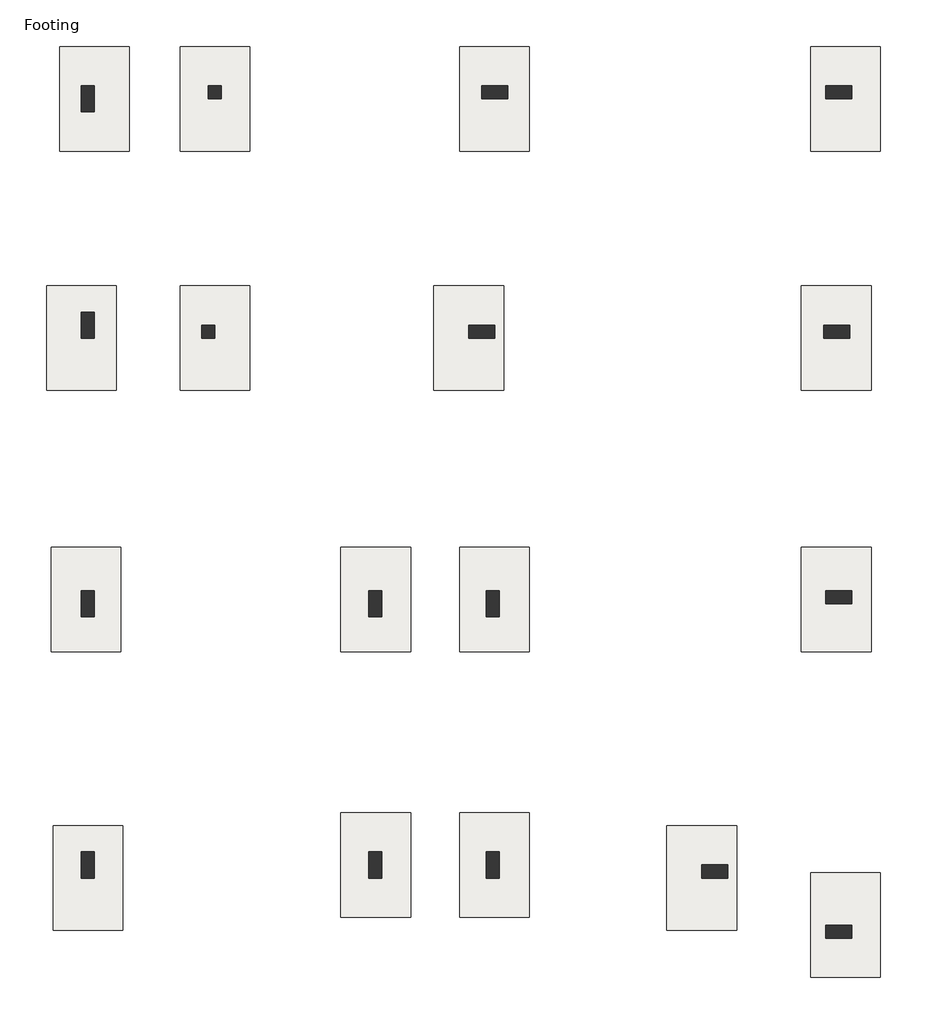
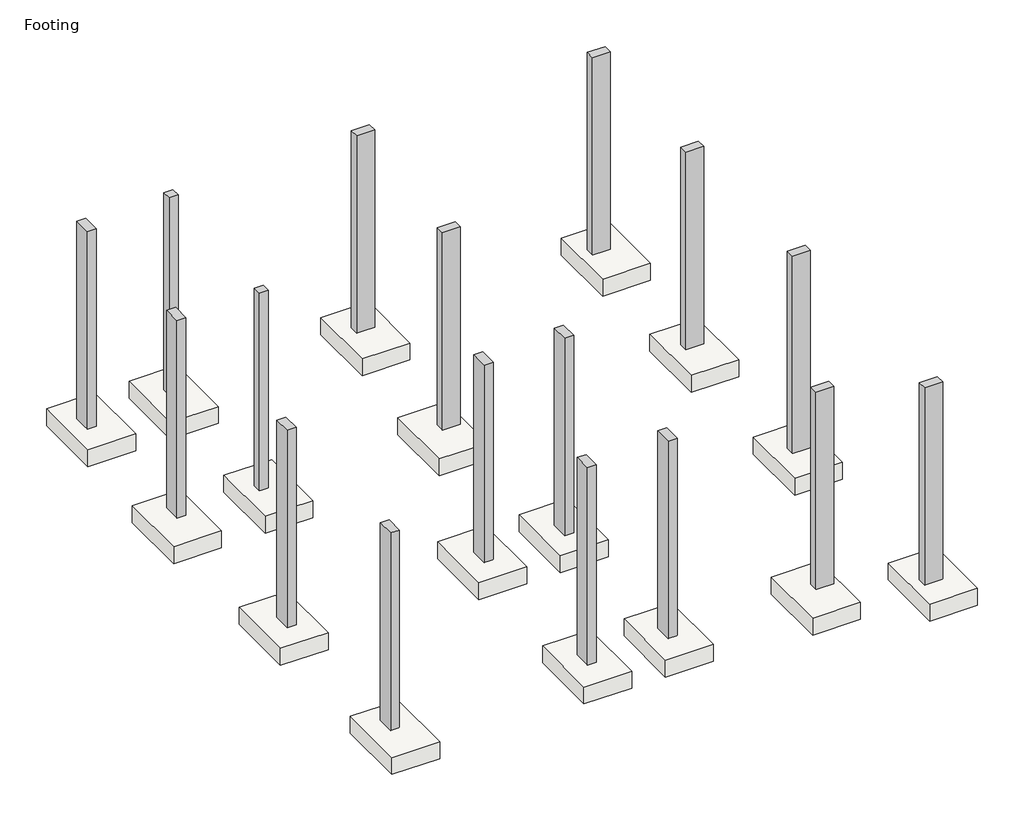
# One storey: 17 columns, 17 slabs.
"""IFC4 building model written with IfcOpenShell, lengths in millimetres."""

from ifc_helpers import new_model, si_unit, frame, origin, place, context, project, spatial, polyline, outline, extrude, faceted_brep, transform, mapped, element, save
from components import slab_5ba74754

model = new_model("IFC4")

# Units and contexts
model_context = context("Model", 3, world=origin())
ifc_project = project(units=[si_unit("LENGTHUNIT", "METRE", prefix="MILLI")], contexts=[model_context])

# Site, building, storey
site = spatial("IfcSite", under=ifc_project)
building = spatial("IfcBuilding", under=site)
storey = spatial("IfcBuildingStorey", under=building, Name="Footing", Elevation=-1828.8)

# Columns
placement = place(None, origin())
element("IfcColumn", 1, ObjectType="Concrete-Rectangular-Column : 9X18", at=placement, inside=storey, context=model_context, shape_type="SweptSolid", body=[
    extrude(outline(polyline([(5601.0916032, 10641.5241878), (5601.0916032, 10184.3241878), (5372.4916032, 10184.3241878), (5372.4916032, 10641.5241878), (5601.0916032, 10641.5241878)])), frame((0.0, 0.0, -1828.8), z_axis=(0.0, 0.0, 1.0), x_axis=(1.0, 0.0, 0.0)), (0.0, 0.0, 1.0), 5334.0),
])
element("IfcColumn", 2, ObjectType="Concrete-Rectangular-Column : 9X18", at=placement, inside=storey, context=model_context, shape_type="SweptSolid", body=[
    extrude(outline(polyline([(5601.0916032, 6679.1241878), (5601.0916032, 6221.9241878), (5372.4916032, 6221.9241878), (5372.4916032, 6679.1241878), (5601.0916032, 6679.1241878)])), frame((0.0, 0.0, -1828.8), z_axis=(0.0, 0.0, 1.0), x_axis=(1.0, 0.0, 0.0)), (0.0, 0.0, 1.0), 5334.0),
])
element("IfcColumn", 3, ObjectType="Concrete-Rectangular-Column : 9X18", at=placement, inside=storey, context=model_context, shape_type="SweptSolid", body=[
    extrude(outline(polyline([(5601.0916032, 1802.3241878), (5601.0916032, 1345.1241878), (5372.4916032, 1345.1241878), (5372.4916032, 1802.3241878), (5601.0916032, 1802.3241878)])), frame((0.0, 0.0, -1828.8), z_axis=(0.0, 0.0, 1.0), x_axis=(1.0, 0.0, 0.0)), (0.0, 0.0, 1.0), 5334.0),
])
element("IfcColumn", 4, ObjectType="Concrete-Rectangular-Column : 9X18", at=placement, inside=storey, context=model_context, shape_type="SweptSolid", body=[
    extrude(outline(polyline([(5601.0916032, -2769.6758122), (5601.0916032, -3226.8758122), (5372.4916032, -3226.8758122), (5372.4916032, -2769.6758122), (5601.0916032, -2769.6758122)])), frame((0.0, 0.0, -1828.8), z_axis=(0.0, 0.0, 1.0), x_axis=(1.0, 0.0, 0.0)), (0.0, 0.0, 1.0), 5334.0),
])
element("IfcColumn", 5, ObjectType="Concrete-Rectangular-Column : 9X18", at=placement, inside=storey, context=model_context, shape_type="SweptSolid", body=[
    extrude(outline(polyline([(10630.2916032, -2769.6758122), (10630.2916032, -3226.8758122), (10401.6916032, -3226.8758122), (10401.6916032, -2769.6758122), (10630.2916032, -2769.6758122)])), frame((0.0, 0.0, -1828.8), z_axis=(0.0, 0.0, 1.0), x_axis=(1.0, 0.0, 0.0)), (0.0, 0.0, 1.0), 5334.0),
])
element("IfcColumn", 6, ObjectType="Concrete-Rectangular-Column : 9X18", at=placement, inside=storey, context=model_context, shape_type="SweptSolid", body=[
    extrude(outline(polyline([(12687.6916032, -2769.6758122), (12687.6916032, -3226.8758122), (12459.0916032, -3226.8758122), (12459.0916032, -2769.6758122), (12687.6916032, -2769.6758122)])), frame((0.0, 0.0, -1828.8), z_axis=(0.0, 0.0, 1.0), x_axis=(1.0, 0.0, 0.0)), (0.0, 0.0, 1.0), 5334.0),
])
element("IfcColumn", 7, ObjectType="Concrete-Rectangular-Column : 9X18", at=placement, inside=storey, context=model_context, shape_type="SweptSolid", body=[
    extrude(outline(polyline([(10630.2916032, 1802.3241878), (10630.2916032, 1345.1241878), (10401.6916032, 1345.1241878), (10401.6916032, 1802.3241878), (10630.2916032, 1802.3241878)])), frame((0.0, 0.0, -1828.8), z_axis=(0.0, 0.0, 1.0), x_axis=(1.0, 0.0, 0.0)), (0.0, 0.0, 1.0), 5334.0),
])
element("IfcColumn", 8, ObjectType="Concrete-Rectangular-Column : 9X18", at=placement, inside=storey, context=model_context, shape_type="Brep", body=[
    faceted_brep([(12687.6916032, 1802.3241878, -1828.8), (12687.6916032, 1345.1241878, -1828.8), (12459.0916032, 1345.1241878, -1828.8), (12459.0916032, 1802.3241878, -1828.8), (12687.6916032, 1802.3241878, 3505.2), (12687.6916032, 1345.1241878, 3505.2), (12459.0916032, 1345.1241878, 3505.2), (12459.0916032, 1802.3241878, 3505.2), (12611.0099466, 1802.3241878, 3505.2)], [[[0, 1, 2, 3]], [[4, 5, 1, 0]], [[5, 6, 2, 1]], [[6, 7, 3, 2]], [[7, 8, 4, 0, 3]], [[4, 8, 7, 6, 5]]]),
])
element("IfcColumn", 9, ObjectType="Concrete-Rectangular-Column : 9X18", at=placement, inside=storey, context=model_context, shape_type="SweptSolid", body=[
    extrude(outline(polyline([(12382.4099466, 10641.5241878), (12839.6099466, 10641.5241878), (12839.6099466, 10412.9241878), (12382.4099466, 10412.9241878), (12382.4099466, 10641.5241878)])), frame((0.0, 0.0, -1828.8), z_axis=(0.0, 0.0, 1.0), x_axis=(1.0, 0.0, 0.0)), (0.0, 0.0, 1.0), 5334.0),
])
element("IfcColumn", 10, ObjectType="Concrete-Rectangular-Column : 9X18", at=placement, inside=storey, context=model_context, shape_type="SweptSolid", body=[
    extrude(outline(polyline([(18402.6916032, 10641.5241878), (18859.8916032, 10641.5241878), (18859.8916032, 10412.9241878), (18402.6916032, 10412.9241878), (18402.6916032, 10641.5241878)])), frame((0.0, 0.0, -1828.8), z_axis=(0.0, 0.0, 1.0), x_axis=(1.0, 0.0, 0.0)), (0.0, 0.0, 1.0), 5334.0),
])
element("IfcColumn", 11, ObjectType="Concrete-Rectangular-Column : 9X18", at=placement, inside=storey, context=model_context, shape_type="Brep", body=[
    faceted_brep([(18366.489508, 6450.5241878, -1828.8), (18823.689508, 6450.5241878, -1828.8), (18823.689508, 6221.9241878, -1828.8), (18366.489508, 6221.9241878, -1828.8), (18366.489508, 6450.5241878, 3505.2), (18402.6916032, 6450.5241878, 3505.2), (18823.689508, 6450.5241878, 3505.2), (18823.689508, 6450.5241878, 3200.4), (18823.689508, 6450.5241878, -152.4), (18823.689508, 6450.5241878, -457.2), (18823.689508, 6221.9241878, 3505.2), (18823.689508, 6221.9241878, 3200.4), (18823.689508, 6221.9241878, -152.4), (18823.689508, 6221.9241878, -457.2), (18402.6916032, 6221.9241878, 3505.2), (18366.489508, 6221.9241878, 3505.2)], [[[0, 1, 2, 3]], [[4, 5, 6, 7, 8, 9, 1, 0]], [[6, 10, 11, 12, 13, 2, 1, 9, 8, 7]], [[10, 14, 15, 3, 2, 13, 12, 11]], [[15, 4, 0, 3]], [[4, 15, 14, 10, 6, 5]]]),
])
element("IfcColumn", 12, ObjectType="Concrete-Rectangular-Column : 9X18", at=placement, inside=storey, context=model_context, shape_type="SweptSolid", body=[
    extrude(outline(polyline([(12153.8099466, 6450.5241878), (12611.0099466, 6450.5241878), (12611.0099466, 6221.9241878), (12153.8099466, 6221.9241878), (12153.8099466, 6450.5241878)])), frame((0.0, 0.0, -1828.8), z_axis=(0.0, 0.0, 1.0), x_axis=(1.0, 0.0, 0.0)), (0.0, 0.0, 1.0), 5334.0),
])
element("IfcColumn", 13, ObjectType="Concrete-Rectangular-Column : 9X18", at=placement, inside=storey, context=model_context, shape_type="Brep", body=[
    faceted_brep([(18402.6916032, 1802.3241878, -1828.8), (18859.8916032, 1802.3241878, -1828.8), (18859.8916032, 1573.7241878, -1828.8), (18402.6916032, 1573.7241878, -1828.8), (18402.6916032, 1802.3241878, 3505.2), (18859.8916032, 1802.3241878, 3505.2), (18859.8916032, 1802.3241878, 3200.4), (18859.8916032, 1802.3241878, -152.4), (18859.8916032, 1802.3241878, -457.2), (18402.6916032, 1802.3241878, -457.2), (18402.6916032, 1802.3241878, -152.4), (18402.6916032, 1802.3241878, 3200.4), (18859.8916032, 1573.7241878, 3505.2), (18859.8916032, 1573.7241878, 3200.4), (18859.8916032, 1573.7241878, -152.4), (18859.8916032, 1573.7241878, -457.2), (18402.6916032, 1573.7241878, 3505.2), (18402.6916032, 1573.7241878, 3200.4), (18402.6916032, 1573.7241878, -152.4), (18402.6916032, 1573.7241878, -457.2)], [[[0, 1, 2, 3]], [[4, 5, 6, 7, 8, 1, 0, 9, 10, 11]], [[5, 12, 13, 14, 15, 2, 1, 8, 7, 6]], [[12, 16, 17, 18, 19, 3, 2, 15, 14, 13]], [[16, 4, 11, 10, 9, 0, 3, 19, 18, 17]], [[4, 16, 12, 5]]]),
])
element("IfcColumn", 14, ObjectType="Concrete-Rectangular-Column : 9X18", at=placement, inside=storey, context=model_context, shape_type="SweptSolid", body=[
    extrude(outline(polyline([(16230.9916032, -2998.2758122), (16688.1916032, -2998.2758122), (16688.1916032, -3226.8758122), (16230.9916032, -3226.8758122), (16230.9916032, -2998.2758122)])), frame((0.0, 0.0, -1828.8), z_axis=(0.0, 0.0, 1.0), x_axis=(1.0, 0.0, 0.0)), (0.0, 0.0, 1.0), 5334.0),
])
element("IfcColumn", 15, ObjectType="Concrete-Rectangular-Column : 9X18", at=placement, inside=storey, context=model_context, shape_type="SweptSolid", body=[
    extrude(outline(polyline([(18402.6916032, -4052.3758122), (18859.8916032, -4052.3758122), (18859.8916032, -4280.9758122), (18402.6916032, -4280.9758122), (18402.6916032, -4052.3758122)])), frame((0.0, 0.0, -1828.8), z_axis=(0.0, 0.0, 1.0), x_axis=(1.0, 0.0, 0.0)), (0.0, 0.0, 1.0), 5334.0),
])
element("IfcColumn", 16, ObjectType="Concrete-Rectangular-Column : 9X9", at=placement, inside=storey, context=model_context, shape_type="Brep", body=[
    faceted_brep([(7708.8099466, 6450.5241878, -1828.8), (7708.8099466, 6221.9241878, -1828.8), (7480.2099466, 6221.9241878, -1828.8), (7480.2099466, 6450.5241878, -1828.8), (7708.8099466, 6450.5241878, 3505.2), (7708.8099466, 6221.9241878, 3505.2), (7708.8099466, 6221.9241878, 3200.4), (7708.8099466, 6221.9241878, -152.4), (7708.8099466, 6221.9241878, -457.2), (7708.8099466, 6450.5241878, -457.2), (7708.8099466, 6450.5241878, -152.4), (7708.8099466, 6450.5241878, 3200.4), (7480.2099466, 6221.9241878, 3505.2), (7480.2099466, 6221.9241878, 3200.4), (7480.2099466, 6221.9241878, -152.4), (7480.2099466, 6221.9241878, -457.2), (7480.2099466, 6450.5241878, 3505.2), (7480.2099466, 6450.5241878, 3200.4), (7480.2099466, 6450.5241878, -152.4), (7480.2099466, 6450.5241878, -457.2)], [[[0, 1, 2, 3]], [[4, 5, 6, 7, 8, 1, 0, 9, 10, 11]], [[5, 12, 13, 14, 15, 2, 1, 8, 7, 6]], [[12, 16, 17, 18, 19, 3, 2, 15, 14, 13]], [[16, 4, 11, 10, 9, 0, 3, 19, 18, 17]], [[4, 16, 12, 5]]]),
])
element("IfcColumn", 17, ObjectType="Concrete-Rectangular-Column : 9X9", at=placement, inside=storey, context=model_context, shape_type="Brep", body=[
    faceted_brep([(7823.1099466, 10641.5241878, -1828.8), (7823.1099466, 10412.9241878, -1828.8), (7594.5099466, 10412.9241878, -1828.8), (7594.5099466, 10641.5241878, -1828.8), (7823.1099466, 10641.5241878, 3505.2), (7823.1099466, 10412.9241878, 3505.2), (7823.1099466, 10412.9241878, 3200.4), (7823.1099466, 10412.9241878, -152.4), (7823.1099466, 10412.9241878, -457.2), (7823.1099466, 10641.5241878, -457.2), (7823.1099466, 10641.5241878, -152.4), (7823.1099466, 10641.5241878, 3200.4), (7594.5099466, 10412.9241878, 3505.2), (7594.5099466, 10412.9241878, 3200.4), (7594.5099466, 10412.9241878, -152.4), (7594.5099466, 10412.9241878, -457.2), (7594.5099466, 10641.5241878, 3505.2), (7594.5099466, 10641.5241878, 3200.4), (7594.5099466, 10641.5241878, -152.4), (7594.5099466, 10641.5241878, -457.2)], [[[0, 1, 2, 3]], [[4, 5, 6, 7, 8, 1, 0, 9, 10, 11]], [[5, 12, 13, 14, 15, 2, 1, 8, 7, 6]], [[12, 16, 17, 18, 19, 3, 2, 15, 14, 13]], [[16, 4, 11, 10, 9, 0, 3, 19, 18, 17]], [[4, 16, 12, 5]]]),
])

# Slabs
slab_shape = slab_5ba74754(model_context)
element("IfcSlab", 18, ObjectType="Footing-Rectangular : 72\" x 48\" x 18\"", at=placement, inside=storey, context=model_context, shape_type="MappedRepresentation", body=[
    mapped(slab_shape, transform((5455.3984765, 1644.7752922, -1828.8), x_axis=(1.0, 0.0, 0.0), y_axis=(0.0, 1.0, 0.0), z_axis=(0.0, 0.0, 1.0))),
])
element("IfcSlab", 19, ObjectType="Footing-Rectangular : 72\" x 48\" x 18\"", at=placement, inside=storey, context=model_context, shape_type="MappedRepresentation", body=[
    mapped(slab_shape, transform((10524.8083528, 1644.7752922, -1828.8), x_axis=(1.0, 0.0, 0.0), y_axis=(0.0, 1.0, 0.0), z_axis=(0.0, 0.0, 1.0))),
])
element("IfcSlab", 20, ObjectType="Footing-Rectangular : 72\" x 48\" x 18\"", at=placement, inside=storey, context=model_context, shape_type="MappedRepresentation", body=[
    mapped(slab_shape, transform((12604.1985426, 1644.7752922, -1828.8), x_axis=(1.0, 0.0, 0.0), y_axis=(0.0, 1.0, 0.0), z_axis=(0.0, 0.0, 1.0))),
])
element("IfcSlab", 21, ObjectType="Footing-Rectangular : 72\" x 48\" x 18\"", at=placement, inside=storey, context=model_context, shape_type="MappedRepresentation", body=[
    mapped(slab_shape, transform((18584.2379158, 1644.7752922, -1828.8), x_axis=(1.0, 0.0, 0.0), y_axis=(0.0, 1.0, 0.0), z_axis=(0.0, 0.0, 1.0))),
])
element("IfcSlab", 22, ObjectType="Footing-Rectangular : 72\" x 48\" x 18\"", at=placement, inside=storey, context=model_context, shape_type="MappedRepresentation", body=[
    mapped(slab_shape, transform((18745.5916032, -4052.3758122, -1828.8), x_axis=(1.0, 0.0, 0.0), y_axis=(0.0, 1.0, 0.0), z_axis=(0.0, 0.0, 1.0))),
])
element("IfcSlab", 23, ObjectType="Footing-Rectangular : 72\" x 48\" x 18\"", at=placement, inside=storey, context=model_context, shape_type="MappedRepresentation", body=[
    mapped(slab_shape, transform((16230.9916032, -3226.8758122, -1828.8), x_axis=(1.0, 0.0, 0.0), y_axis=(0.0, 1.0, 0.0), z_axis=(0.0, 0.0, 1.0))),
])
element("IfcSlab", 24, ObjectType="Footing-Rectangular : 72\" x 48\" x 18\"", at=placement, inside=storey, context=model_context, shape_type="MappedRepresentation", body=[
    mapped(slab_shape, transform((12604.1985426, -2998.2758122, -1828.8), x_axis=(1.0, 0.0, 0.0), y_axis=(0.0, 1.0, 0.0), z_axis=(0.0, 0.0, 1.0))),
])
element("IfcSlab", 25, ObjectType="Footing-Rectangular : 72\" x 48\" x 18\"", at=placement, inside=storey, context=model_context, shape_type="MappedRepresentation", body=[
    mapped(slab_shape, transform((10524.8083528, -2998.2758122, -1828.8), x_axis=(1.0, 0.0, 0.0), y_axis=(0.0, 1.0, 0.0), z_axis=(0.0, 0.0, 1.0))),
])
element("IfcSlab", 26, ObjectType="Footing-Rectangular : 72\" x 48\" x 18\"", at=placement, inside=storey, context=model_context, shape_type="MappedRepresentation", body=[
    mapped(slab_shape, transform((5486.7916032, -3226.8758122, -1828.8), x_axis=(1.0, 0.0, 0.0), y_axis=(0.0, 1.0, 0.0), z_axis=(0.0, 0.0, 1.0))),
])
element("IfcSlab", 27, ObjectType="Footing-Rectangular : 72\" x 48\" x 18\"", at=placement, inside=storey, context=model_context, shape_type="MappedRepresentation", body=[
    mapped(slab_shape, transform((5372.4916032, 6221.9241878, -1828.8), x_axis=(1.0, 0.0, 0.0), y_axis=(0.0, 1.0, 0.0), z_axis=(0.0, 0.0, 1.0))),
])
element("IfcSlab", 28, ObjectType="Footing-Rectangular : 72\" x 48\" x 18\"", at=placement, inside=storey, context=model_context, shape_type="MappedRepresentation", body=[
    mapped(slab_shape, transform((7708.8099466, 6221.9241878, -1828.8), x_axis=(1.0, 0.0, 0.0), y_axis=(0.0, 1.0, 0.0), z_axis=(0.0, 0.0, 1.0))),
])
element("IfcSlab", 29, ObjectType="Footing-Rectangular : 72\" x 48\" x 18\"", at=placement, inside=storey, context=model_context, shape_type="MappedRepresentation", body=[
    mapped(slab_shape, transform((12153.8099466, 6221.9241878, -1828.8), x_axis=(1.0, 0.0, 0.0), y_axis=(0.0, 1.0, 0.0), z_axis=(0.0, 0.0, 1.0))),
])
element("IfcSlab", 30, ObjectType="Footing-Rectangular : 72\" x 48\" x 18\"", at=placement, inside=storey, context=model_context, shape_type="MappedRepresentation", body=[
    mapped(slab_shape, transform((18584.2379158, 6221.9241878, -1828.8), x_axis=(1.0, 0.0, 0.0), y_axis=(0.0, 1.0, 0.0), z_axis=(0.0, 0.0, 1.0))),
])
element("IfcSlab", 31, ObjectType="Footing-Rectangular : 72\" x 48\" x 18\"", at=placement, inside=storey, context=model_context, shape_type="MappedRepresentation", body=[
    mapped(slab_shape, transform((18745.5916032, 10412.9241878, -1828.8), x_axis=(1.0, 0.0, 0.0), y_axis=(0.0, 1.0, 0.0), z_axis=(0.0, 0.0, 1.0))),
])
element("IfcSlab", 32, ObjectType="Footing-Rectangular : 72\" x 48\" x 18\"", at=placement, inside=storey, context=model_context, shape_type="MappedRepresentation", body=[
    mapped(slab_shape, transform((12604.1985426, 10412.9241878, -1828.8), x_axis=(1.0, 0.0, 0.0), y_axis=(0.0, 1.0, 0.0), z_axis=(0.0, 0.0, 1.0))),
])
element("IfcSlab", 33, ObjectType="Footing-Rectangular : 72\" x 48\" x 18\"", at=placement, inside=storey, context=model_context, shape_type="MappedRepresentation", body=[
    mapped(slab_shape, transform((7708.8099466, 10412.9241878, -1828.8), x_axis=(1.0, 0.0, 0.0), y_axis=(0.0, 1.0, 0.0), z_axis=(0.0, 0.0, 1.0))),
])
element("IfcSlab", 34, ObjectType="Footing-Rectangular : 72\" x 48\" x 18\"", at=placement, inside=storey, context=model_context, shape_type="MappedRepresentation", body=[
    mapped(slab_shape, transform((5601.0916032, 10412.9241878, -1828.8), x_axis=(1.0, 0.0, 0.0), y_axis=(0.0, 1.0, 0.0), z_axis=(0.0, 0.0, 1.0))),
])

save(model, "model.ifc")

# Revit data of these elements
# Type "Concrete-Rectangular-Column : 9X18"
#   Assembly Code = "B10"
#   b = 0' - 9"
#   h = 1' - 6"
#   Structural Material [instance default] = Concrete, Cast-in-Place gray
# Type "Concrete-Rectangular-Column : 9X9"
#   Assembly Code = "B10"
#   b = 0' - 9"
#   h = 0' - 9"
#   Structural Material [instance default] = Concrete, Cast-in-Place gray
# Type "Footing-Rectangular : 72\" x 48\" x 18\""
#   Assembly Code = "A1010100"
#   Width = 4' - 0"
#   Length = 6' - 0"
#   Foundation Thickness = 1' - 6"
#   Structural Material [instance default] = Concrete, Cast-in-Place gray
# Elements 1, 2, 3, 4, 5, 6, 7, 8, 9, 10, 11, 12, 13, 14, 15 (IfcColumn, "Concrete-Rectangular-Column : 9X18")
#   Structural Material = Concrete, Cast-in-Place gray
#   Phase Created = A10 - Substructure
#   Materials on its faces: "Concrete, Cast-in-Place gray"
# Elements 16, 17 (IfcColumn, "Concrete-Rectangular-Column : 9X9")
#   Structural Material = Concrete, Cast-in-Place gray
#   Phase Created = A10 - Substructure
#   Materials on its faces: "Concrete, Cast-in-Place gray"
# Elements 18, 19, 20, 21, 22, 23, 24, 25, 26, 27, 28, 29, 30, 31, 32, 33, 34 (IfcSlab, "Footing-Rectangular : 72\" x 48\" x 18\"")
#   Structural Material = Concrete, Cast-in-Place gray
#   Phase Created = A10 - Substructure
#   Materials on its faces: "Concrete, Cast-in-Place gray"
# Materials
#   "Concrete, Cast-in-Place gray": class "Concrete", colour RGB 192 192 192, transparency 0, Description = "Cast-in-place concrete", Cost = 0
